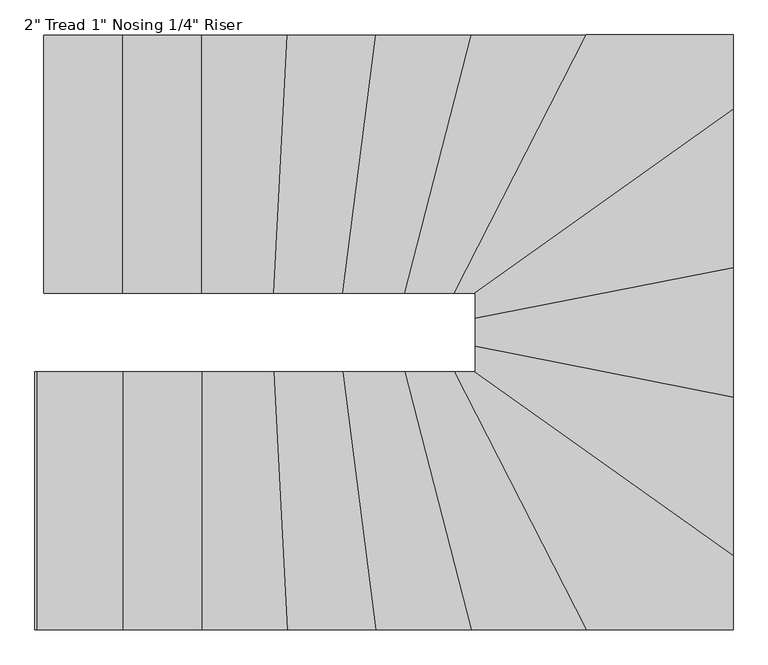
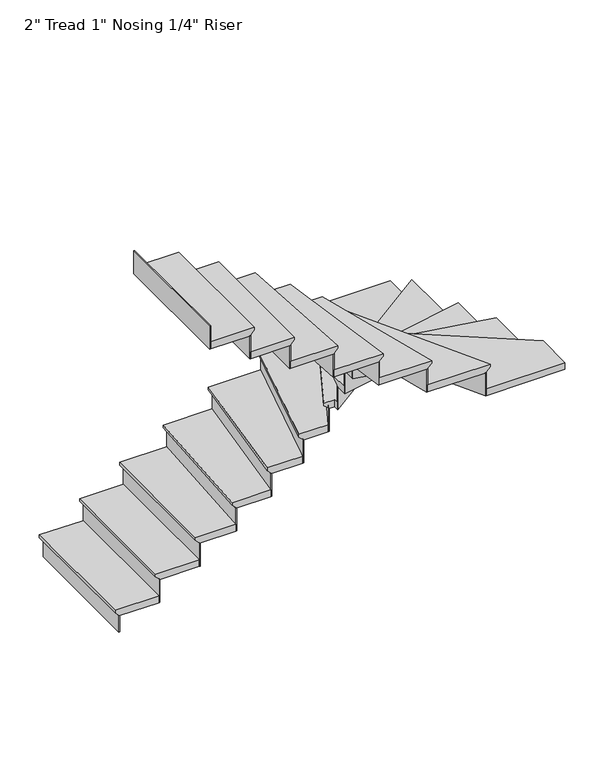
"""IFC4 building model written with IfcOpenShell, lengths in millimetres: stair flight geometry."""

from ifc_helpers import new_model, si_unit, origin, place, context, project, spatial, faceted_brep, source, transform, mapped, element, save


def stair_flight_cbf97d32(model_context):
    return source(origin(), model_context, "Body", "Brep", [
        faceted_brep([(-7803.5154882, 6201.5759458, 150.2833333), (-7803.5154882, 6201.5759458, 169.3333333), (-7803.5154882, 7115.9759458, 169.3333333), (-7803.5154882, 7115.9759458, 150.2833333), (-7778.1154882, 6201.5759458, 124.8833333), (-7778.1154882, 7115.9759458, 124.8833333), (-7498.7154882, 6201.5759458, 169.3333333), (-7498.7154882, 7115.9759458, 169.3333333), (-7778.1154882, 7115.9759458, 118.5333333), (-7498.7154882, 7115.9759458, 118.5333333), (-7498.7154882, 6201.5759458, 118.5333333), (-7778.1154882, 6201.5759458, 118.5333333)], [[[0, 1, 2, 3]], [[4, 0, 3, 5]], [[2, 1, 6, 7]], [[8, 9, 10, 11]], [[2, 7, 9, 8, 5, 3]], [[8, 11, 4, 5]], [[6, 1, 0, 4, 11, 10]], [[7, 6, 10, 9]]]),
        faceted_brep([(-7778.1154882, 6201.5759458, 118.5333333), (-7778.1154882, 6201.5759458, 0.0), (-7771.7654882, 6201.5759458, 0.0), (-7771.7654882, 6201.5759458, 118.5333333), (-7778.1154882, 7115.9759458, 118.5333333), (-7771.7654882, 7115.9759458, 118.5333333), (-7771.7654882, 7115.9759458, 0.0), (-7778.1154882, 7115.9759458, 0.0)], [[[0, 1, 2, 3]], [[4, 5, 6, 7]], [[1, 0, 4, 7]], [[2, 1, 7, 6]], [[3, 2, 6, 5]], [[0, 3, 5, 4]]]),
        faceted_brep([(-7498.7154882, 6201.5759458, 287.8666667), (-7498.7154882, 6201.5759458, 118.5333333), (-7492.3654882, 6201.5759458, 118.5333333), (-7492.3654882, 6201.5759458, 287.8666667), (-7498.7154882, 7115.9759458, 287.8666667), (-7492.3654882, 7115.9759458, 287.8666667), (-7492.3654882, 7115.9759458, 118.5333333), (-7498.7154882, 7115.9759458, 118.5333333)], [[[0, 1, 2, 3]], [[4, 5, 6, 7]], [[1, 0, 4, 7]], [[2, 1, 7, 6]], [[3, 2, 6, 5]], [[0, 3, 5, 4]]]),
        faceted_brep([(-7524.1154882, 7115.9759458, 338.6666667), (-7524.1154882, 6201.5759458, 338.6666667), (-7219.3154882, 6201.5759458, 338.6666667), (-7219.3154882, 7115.9759458, 338.6666667), (-7498.7154882, 7115.9759458, 287.8666667), (-7219.3154882, 7115.9759458, 287.8666667), (-7219.3154882, 6201.5759458, 287.8666667), (-7498.7154882, 6201.5759458, 287.8666667), (-7498.7154882, 7115.9759458, 294.2166667), (-7524.1154882, 7115.9759458, 319.6166667), (-7498.7154882, 6201.5759458, 294.2166667), (-7524.1154882, 6201.5759458, 319.6166667)], [[[0, 1, 2, 3]], [[4, 5, 6, 7]], [[0, 3, 5, 4, 8, 9]], [[4, 7, 10, 8]], [[2, 1, 11, 10, 7, 6]], [[3, 2, 6, 5]], [[11, 1, 0, 9]], [[10, 11, 9, 8]]]),
        faceted_brep([(-7219.3154882, 6201.5759458, 457.2), (-7219.3154882, 6201.5759458, 287.8666667), (-7212.9654882, 6201.5759458, 287.8666667), (-7212.9654882, 6201.5759458, 457.2), (-7219.3154882, 7115.9759458, 457.2), (-7212.9654882, 7115.9759458, 457.2), (-7212.9654882, 7115.9759458, 287.8666667), (-7219.3154882, 7115.9759458, 287.8666667)], [[[0, 1, 2, 3]], [[4, 5, 6, 7]], [[1, 0, 4, 7]], [[2, 1, 7, 6]], [[3, 2, 6, 5]], [[0, 3, 5, 4]]]),
        faceted_brep([(-7244.7154882, 7115.9759458, 508.0), (-7244.7154882, 6201.5759458, 508.0), (-6963.6483268, 6201.5759458, 508.0), (-6916.1140564, 7115.9759458, 508.0), (-7219.3154882, 7115.9759458, 457.2), (-6916.1140564, 7115.9759458, 457.2), (-6963.6483268, 6201.5759458, 457.2), (-7219.3154882, 6201.5759458, 457.2), (-7219.3154882, 7115.9759458, 463.55), (-7244.7154882, 7115.9759458, 488.95), (-7219.3154882, 6201.5759458, 463.55), (-7244.7154882, 6201.5759458, 488.95)], [[[0, 1, 2, 3]], [[4, 5, 6, 7]], [[0, 3, 5, 4, 8, 9]], [[4, 7, 10, 8]], [[2, 1, 11, 10, 7, 6]], [[3, 2, 6, 5]], [[11, 1, 0, 9]], [[10, 11, 9, 8]]]),
        faceted_brep([(-6963.6483268, 6201.5759458, 626.5333333), (-6963.6483268, 6201.5759458, 457.2), (-6957.2897526, 6201.5759458, 457.2), (-6957.2897526, 6201.5759458, 626.5333333), (-6916.1140564, 7115.9759458, 626.5333333), (-6909.7554822, 7115.9759458, 626.5333333), (-6909.7554822, 7115.9759458, 457.2), (-6916.1140564, 7115.9759458, 457.2)], [[[0, 1, 2, 3]], [[4, 5, 6, 7]], [[1, 0, 4, 7]], [[2, 1, 7, 6]], [[3, 2, 6, 5]], [[0, 3, 5, 4]]]),
        faceted_brep([(-6941.548353, 7115.9759458, 677.3333333), (-6989.0826234, 6201.5759458, 677.3333333), (-6719.4816269, 6201.5759458, 677.3333333), (-6601.1255753, 7115.9759458, 677.3333333), (-6916.1140564, 7115.9759458, 626.5333333), (-6601.1255753, 7115.9759458, 626.5333333), (-6719.4816269, 6201.5759458, 626.5333333), (-6963.6483268, 6201.5759458, 626.5333333), (-6916.1140564, 7115.9759458, 632.8833333), (-6941.548353, 7115.9759458, 658.2833333), (-6963.6483268, 6201.5759458, 632.8833333), (-6989.0826234, 6201.5759458, 658.2833333)], [[[0, 1, 2, 3]], [[4, 5, 6, 7]], [[0, 3, 5, 4, 8, 9]], [[4, 7, 10, 8]], [[2, 1, 11, 10, 7, 6]], [[3, 2, 6, 5]], [[11, 1, 0, 9]], [[10, 11, 9, 8]]]),
        faceted_brep([(-6719.4816269, 6201.5759458, 795.8666667), (-6719.4816269, 6201.5759458, 626.5333333), (-6713.0786552, 6201.5759458, 626.5333333), (-6713.0786552, 6201.5759458, 795.8666667), (-6601.1255753, 7115.9759458, 795.8666667), (-6594.7226035, 7115.9759458, 795.8666667), (-6594.7226035, 7115.9759458, 626.5333333), (-6601.1255753, 7115.9759458, 626.5333333)], [[[0, 1, 2, 3]], [[4, 5, 6, 7]], [[1, 0, 4, 7]], [[2, 1, 7, 6]], [[3, 2, 6, 5]], [[0, 3, 5, 4]]]),
        faceted_brep([(-6626.7374624, 7115.9759458, 846.6666667), (-6745.0935141, 6201.5759458, 846.6666667), (-6497.8544045, 6201.5759458, 846.6666667), (-6262.7239571, 7115.9759458, 846.6666667), (-6601.1255753, 7115.9759458, 795.8666667), (-6262.7239571, 7115.9759458, 795.8666667), (-6497.8544045, 6201.5759458, 795.8666667), (-6719.4816269, 6201.5759458, 795.8666667), (-6601.1255753, 7115.9759458, 802.2166667), (-6626.7374624, 7115.9759458, 827.6166667), (-6719.4816269, 6201.5759458, 802.2166667), (-6745.0935141, 6201.5759458, 827.6166667)], [[[0, 1, 2, 3]], [[4, 5, 6, 7]], [[0, 3, 5, 4, 8, 9]], [[4, 7, 10, 8]], [[2, 1, 11, 10, 7, 6]], [[3, 2, 6, 5]], [[11, 1, 0, 9]], [[10, 11, 9, 8]]]),
        faceted_brep([(-6497.8544045, 6201.5759458, 965.2), (-6497.8544045, 6201.5759458, 795.8666667), (-6491.2978276, 6201.5759458, 795.8666667), (-6491.2978276, 6201.5759458, 965.2), (-6262.7239571, 7115.9759458, 965.2), (-6256.1673802, 7115.9759458, 965.2), (-6256.1673802, 7115.9759458, 795.8666667), (-6262.7239571, 7115.9759458, 795.8666667)], [[[0, 1, 2, 3]], [[4, 5, 6, 7]], [[1, 0, 4, 7]], [[2, 1, 7, 6]], [[3, 2, 6, 5]], [[0, 3, 5, 4]]]),
        faceted_brep([(-6288.9502645, 7115.9759458, 1016.0), (-6524.0807119, 6201.5759458, 1016.0), (-6321.5077684, 6201.5759458, 1016.0), (-5852.6831471, 7115.9759458, 1016.0), (-6262.7239571, 7115.9759458, 965.2), (-5852.6831471, 7115.9759458, 965.2), (-6321.5077684, 6201.5759458, 965.2), (-6497.8544045, 6201.5759458, 965.2), (-6262.7239571, 7115.9759458, 971.55), (-6288.9502645, 7115.9759458, 996.95), (-6497.8544045, 6201.5759458, 971.55), (-6524.0807119, 6201.5759458, 996.95)], [[[0, 1, 2, 3]], [[4, 5, 6, 7]], [[0, 3, 5, 4, 8, 9]], [[4, 7, 10, 8]], [[2, 1, 11, 10, 7, 6]], [[3, 2, 6, 5]], [[11, 1, 0, 9]], [[10, 11, 9, 8]]]),
        faceted_brep([(-6321.5077684, 6201.5759458, 1134.5333333), (-6321.5077684, 6201.5759458, 965.2), (-6314.3717853, 6201.5759458, 965.2), (-6314.3717853, 6201.5759458, 1134.5333333), (-5852.6831471, 7115.9759458, 1134.5333333), (-5845.5471639, 7115.9759458, 1134.5333333), (-5845.5471639, 7115.9759458, 965.2), (-5852.6831471, 7115.9759458, 965.2)], [[[0, 1, 2, 3]], [[4, 5, 6, 7]], [[1, 0, 4, 7]], [[2, 1, 7, 6]], [[3, 2, 6, 5]], [[0, 3, 5, 4]]]),
        faceted_brep([(-5361.3837964, 6822.2948121, 1185.3333333), (-5361.3837964, 7115.9759458, 1185.3333333), (-5881.2270796, 7115.9759458, 1185.3333333), (-6350.0517009, 6201.5759458, 1185.3333333), (-6275.7837964, 6201.5759458, 1185.3333333), (-6275.7837964, 6172.020863, 1185.3333333), (-5361.3837964, 7115.9759458, 1134.5333333), (-5361.3837964, 6822.2948121, 1134.5333333), (-6275.7837964, 6172.020863, 1134.5333333), (-6275.7837964, 6201.5759458, 1134.5333333), (-6321.5077684, 6201.5759458, 1134.5333333), (-5852.6831471, 7115.9759458, 1134.5333333), (-5852.6831471, 7115.9759458, 1140.8833333), (-5881.2270796, 7115.9759458, 1166.2833333), (-6321.5077684, 6201.5759458, 1140.8833333), (-6350.0517009, 6201.5759458, 1166.2833333)], [[[0, 1, 2, 3, 4, 5]], [[6, 7, 8, 9, 10, 11]], [[1, 0, 7, 6]], [[2, 1, 6, 11, 12, 13]], [[11, 10, 14, 12]], [[4, 3, 15, 14, 10, 9]], [[5, 4, 9, 8]], [[0, 5, 8, 7]], [[15, 3, 2, 13]], [[14, 15, 13, 12]]]),
        faceted_brep([(-6275.7837964, 6172.020863, 1303.8666667), (-6275.7837964, 6172.020863, 1134.5333333), (-6275.7837964, 6164.2288882, 1134.5333333), (-6275.7837964, 6164.2288882, 1303.8666667), (-5361.3837964, 6822.2948121, 1303.8666667), (-5361.3837964, 6814.5028373, 1303.8666667), (-5361.3837964, 6814.5028373, 1134.5333333), (-5361.3837964, 6822.2948121, 1134.5333333)], [[[0, 1, 2, 3]], [[4, 5, 6, 7]], [[1, 0, 4, 7]], [[2, 1, 7, 6]], [[3, 2, 6, 5]], [[0, 3, 5, 4]]]),
        faceted_brep([(-5361.3837964, 6853.4627113, 1354.6666667), (-6275.7837964, 6203.1887621, 1354.6666667), (-6275.7837964, 6085.5667759, 1354.6666667), (-5361.3837964, 6265.8076322, 1354.6666667), (-5361.3837964, 6822.2948121, 1303.8666667), (-5361.3837964, 6265.8076322, 1303.8666667), (-6275.7837964, 6085.5667759, 1303.8666667), (-6275.7837964, 6172.020863, 1303.8666667), (-5361.3837964, 6822.2948121, 1310.2166667), (-5361.3837964, 6853.4627113, 1335.6166667), (-6275.7837964, 6172.020863, 1310.2166667), (-6275.7837964, 6203.1887621, 1335.6166667)], [[[0, 1, 2, 3]], [[4, 5, 6, 7]], [[0, 3, 5, 4, 8, 9]], [[4, 7, 10, 8]], [[2, 1, 11, 10, 7, 6]], [[3, 2, 6, 5]], [[11, 1, 0, 9]], [[10, 11, 9, 8]]]),
        faceted_brep([(-6275.7837964, 6085.5667759, 1473.2), (-6275.7837964, 6085.5667759, 1303.8666667), (-6275.7837964, 6079.0945905, 1303.8666667), (-6275.7837964, 6079.0945905, 1473.2), (-5361.3837964, 6265.8076322, 1473.2), (-5361.3837964, 6259.3354468, 1473.2), (-5361.3837964, 6259.3354468, 1303.8666667), (-5361.3837964, 6265.8076322, 1303.8666667)], [[[0, 1, 2, 3]], [[4, 5, 6, 7]], [[1, 0, 4, 7]], [[2, 1, 7, 6]], [[3, 2, 6, 5]], [[0, 3, 5, 4]]]),
        faceted_brep([(-5361.3837964, 6291.696374, 1524.0), (-6275.7837964, 6111.4555176, 1524.0), (-6275.7837964, 5986.4076322, 1524.0), (-5361.3837964, 5806.1667759, 1524.0), (-5361.3837964, 6265.8076322, 1473.2), (-5361.3837964, 5806.1667759, 1473.2), (-6275.7837964, 5986.4076322, 1473.2), (-6275.7837964, 6085.5667759, 1473.2), (-5361.3837964, 6265.8076322, 1479.55), (-5361.3837964, 6291.696374, 1504.95), (-6275.7837964, 6085.5667759, 1479.55), (-6275.7837964, 6111.4555176, 1504.95)], [[[0, 1, 2, 3]], [[4, 5, 6, 7]], [[0, 3, 5, 4, 8, 9]], [[4, 7, 10, 8]], [[2, 1, 11, 10, 7, 6]], [[3, 2, 6, 5]], [[11, 1, 0, 9]], [[10, 11, 9, 8]]]),
        faceted_brep([(-6275.7837964, 5986.4076322, 1642.5333333), (-6275.7837964, 5986.4076322, 1473.2), (-6275.7837964, 5979.9354468, 1473.2), (-6275.7837964, 5979.9354468, 1642.5333333), (-5361.3837964, 5806.1667759, 1642.5333333), (-5361.3837964, 5799.6945905, 1642.5333333), (-5361.3837964, 5799.6945905, 1473.2), (-5361.3837964, 5806.1667759, 1473.2)], [[[0, 1, 2, 3]], [[4, 5, 6, 7]], [[1, 0, 4, 7]], [[2, 1, 7, 6]], [[3, 2, 6, 5]], [[0, 3, 5, 4]]]),
        faceted_brep([(-5361.3837964, 5832.0555176, 1693.3333333), (-6275.7837964, 6012.296374, 1693.3333333), (-6275.7837964, 5922.1759458, 1693.3333333), (-6321.8792709, 5922.1759458, 1693.3333333), (-5361.3837964, 5239.1212812, 1693.3333333), (-5361.3837964, 5806.1667759, 1642.5333333), (-5361.3837964, 5239.1212812, 1642.5333333), (-6321.8792709, 5922.1759458, 1642.5333333), (-6275.7837964, 5922.1759458, 1642.5333333), (-6275.7837964, 5986.4076322, 1642.5333333), (-5361.3837964, 5806.1667759, 1648.8833333), (-5361.3837964, 5832.0555176, 1674.2833333), (-6275.7837964, 5986.4076322, 1648.8833333), (-6275.7837964, 6012.296374, 1674.2833333)], [[[0, 1, 2, 3, 4]], [[5, 6, 7, 8, 9]], [[0, 4, 6, 5, 10, 11]], [[5, 9, 12, 10]], [[2, 1, 13, 12, 9, 8]], [[3, 2, 8, 7]], [[4, 3, 7, 6]], [[13, 1, 0, 11]], [[12, 13, 11, 10]]]),
        faceted_brep([(-6321.8792709, 5922.1759458, 1811.8666667), (-6321.8792709, 5922.1759458, 1642.5333333), (-6332.8361634, 5922.1759458, 1642.5333333), (-6332.8361634, 5922.1759458, 1811.8666667), (-5361.3837964, 5239.1212812, 1811.8666667), (-5361.3837964, 5231.3293064, 1811.8666667), (-5361.3837964, 5231.3293064, 1642.5333333), (-5361.3837964, 5239.1212812, 1642.5333333)], [[[0, 1, 2, 3]], [[4, 5, 6, 7]], [[1, 0, 4, 7]], [[2, 1, 7, 6]], [[3, 2, 6, 5]], [[0, 3, 5, 4]]]),
        faceted_brep([(-5909.7710121, 5007.7759458, 1862.6666667), (-5361.3837964, 5007.7759458, 1862.6666667), (-5361.3837964, 5270.2891803, 1862.6666667), (-6278.0517009, 5922.1759458, 1862.6666667), (-6378.5956335, 5922.1759458, 1862.6666667), (-5361.3837964, 5007.7759458, 1811.8666667), (-5909.7710121, 5007.7759458, 1811.8666667), (-6378.5956335, 5922.1759458, 1811.8666667), (-6321.8792709, 5922.1759458, 1811.8666667), (-5361.3837964, 5239.1212812, 1811.8666667), (-5361.3837964, 5239.1212812, 1818.2166667), (-5361.3837964, 5270.2891803, 1843.6166667), (-6321.8792709, 5922.1759458, 1818.2166667), (-6278.0517009, 5922.1759458, 1843.6166667)], [[[0, 1, 2, 3, 4]], [[5, 6, 7, 8, 9]], [[1, 0, 6, 5]], [[2, 1, 5, 9, 10, 11]], [[9, 8, 12, 10]], [[4, 3, 13, 12, 8, 7]], [[0, 4, 7, 6]], [[13, 3, 2, 11]], [[12, 13, 11, 10]]]),
        faceted_brep([(-6378.5956335, 5922.1759458, 1981.2), (-6378.5956335, 5922.1759458, 1811.8666667), (-6385.7316166, 5922.1759458, 1811.8666667), (-6385.7316166, 5922.1759458, 1981.2), (-5909.7710121, 5007.7759458, 1981.2), (-5916.9069953, 5007.7759458, 1981.2), (-5916.9069953, 5007.7759458, 1811.8666667), (-5909.7710121, 5007.7759458, 1811.8666667)], [[[0, 1, 2, 3]], [[4, 5, 6, 7]], [[1, 0, 4, 7]], [[2, 1, 7, 6]], [[3, 2, 6, 5]], [[0, 3, 5, 4]]]),
        faceted_brep([(-5881.2270796, 5007.7759458, 2032.0), (-6350.0517009, 5922.1759458, 2032.0), (-6550.3070194, 5922.1759458, 2032.0), (-6315.176572, 5007.7759458, 2032.0), (-5909.7710121, 5007.7759458, 1981.2), (-6315.176572, 5007.7759458, 1981.2), (-6550.3070194, 5922.1759458, 1981.2), (-6378.5956335, 5922.1759458, 1981.2), (-5909.7710121, 5007.7759458, 1987.55), (-5881.2270796, 5007.7759458, 2012.95), (-6378.5956335, 5922.1759458, 1987.55), (-6350.0517009, 5922.1759458, 2012.95)], [[[0, 1, 2, 3]], [[4, 5, 6, 7]], [[0, 3, 5, 4, 8, 9]], [[4, 7, 10, 8]], [[2, 1, 11, 10, 7, 6]], [[3, 2, 6, 5]], [[11, 1, 0, 9]], [[10, 11, 9, 8]]]),
        faceted_brep([(-6550.3070194, 5922.1759458, 2150.5333333), (-6550.3070194, 5922.1759458, 1981.2), (-6556.8635963, 5922.1759458, 1981.2), (-6556.8635963, 5922.1759458, 2150.5333333), (-6315.176572, 5007.7759458, 2150.5333333), (-6321.7331489, 5007.7759458, 2150.5333333), (-6321.7331489, 5007.7759458, 1981.2), (-6315.176572, 5007.7759458, 1981.2)], [[[0, 1, 2, 3]], [[4, 5, 6, 7]], [[1, 0, 4, 7]], [[2, 1, 7, 6]], [[3, 2, 6, 5]], [[0, 3, 5, 4]]]),
        faceted_brep([(-6288.9502645, 5007.7759458, 2201.3333333), (-6524.0807119, 5922.1759458, 2201.3333333), (-6770.7054012, 5922.1759458, 2201.3333333), (-6652.3493495, 5007.7759458, 2201.3333333), (-6315.176572, 5007.7759458, 2150.5333333), (-6652.3493495, 5007.7759458, 2150.5333333), (-6770.7054012, 5922.1759458, 2150.5333333), (-6550.3070194, 5922.1759458, 2150.5333333), (-6315.176572, 5007.7759458, 2156.8833333), (-6288.9502645, 5007.7759458, 2182.2833333), (-6550.3070194, 5922.1759458, 2156.8833333), (-6524.0807119, 5922.1759458, 2182.2833333)], [[[0, 1, 2, 3]], [[4, 5, 6, 7]], [[0, 3, 5, 4, 8, 9]], [[4, 7, 10, 8]], [[2, 1, 11, 10, 7, 6]], [[3, 2, 6, 5]], [[11, 1, 0, 9]], [[10, 11, 9, 8]]]),
        faceted_brep([(-6770.7054012, 5922.1759458, 2319.8666667), (-6770.7054012, 5922.1759458, 2150.5333333), (-6777.108373, 5922.1759458, 2150.5333333), (-6777.108373, 5922.1759458, 2319.8666667), (-6652.3493495, 5007.7759458, 2319.8666667), (-6658.7523213, 5007.7759458, 2319.8666667), (-6658.7523213, 5007.7759458, 2150.5333333), (-6652.3493495, 5007.7759458, 2150.5333333)], [[[0, 1, 2, 3]], [[4, 5, 6, 7]], [[1, 0, 4, 7]], [[2, 1, 7, 6]], [[3, 2, 6, 5]], [[0, 3, 5, 4]]]),
        faceted_brep([(-6626.7374624, 5007.7759458, 2370.6666667), (-6745.0935141, 5922.1759458, 2370.6666667), (-7014.5169201, 5922.1759458, 2370.6666667), (-6966.9826497, 5007.7759458, 2370.6666667), (-6652.3493495, 5007.7759458, 2319.8666667), (-6966.9826497, 5007.7759458, 2319.8666667), (-7014.5169201, 5922.1759458, 2319.8666667), (-6770.7054012, 5922.1759458, 2319.8666667), (-6652.3493495, 5007.7759458, 2326.2166667), (-6626.7374624, 5007.7759458, 2351.6166667), (-6770.7054012, 5922.1759458, 2326.2166667), (-6745.0935141, 5922.1759458, 2351.6166667)], [[[0, 1, 2, 3]], [[4, 5, 6, 7]], [[0, 3, 5, 4, 8, 9]], [[4, 7, 10, 8]], [[2, 1, 11, 10, 7, 6]], [[3, 2, 6, 5]], [[11, 1, 0, 9]], [[10, 11, 9, 8]]]),
        faceted_brep([(-7014.5169201, 5922.1759458, 2489.2), (-7014.5169201, 5922.1759458, 2319.8666667), (-7020.8754943, 5922.1759458, 2319.8666667), (-7020.8754943, 5922.1759458, 2489.2), (-6966.9826497, 5007.7759458, 2489.2), (-6973.3412239, 5007.7759458, 2489.2), (-6973.3412239, 5007.7759458, 2319.8666667), (-6966.9826497, 5007.7759458, 2319.8666667)], [[[0, 1, 2, 3]], [[4, 5, 6, 7]], [[1, 0, 4, 7]], [[2, 1, 7, 6]], [[3, 2, 6, 5]], [[0, 3, 5, 4]]]),
        faceted_brep([(-6941.548353, 5007.7759458, 2540.0), (-6989.0826234, 5922.1759458, 2540.0), (-7270.1154882, 5922.1759458, 2540.0), (-7270.1154882, 5007.7759458, 2540.0), (-6966.9826497, 5007.7759458, 2489.2), (-7270.1154882, 5007.7759458, 2489.2), (-7270.1154882, 5922.1759458, 2489.2), (-7014.5169201, 5922.1759458, 2489.2), (-6966.9826497, 5007.7759458, 2495.55), (-6941.548353, 5007.7759458, 2520.95), (-7014.5169201, 5922.1759458, 2495.55), (-6989.0826234, 5922.1759458, 2520.95)], [[[0, 1, 2, 3]], [[4, 5, 6, 7]], [[0, 3, 5, 4, 8, 9]], [[4, 7, 10, 8]], [[2, 1, 11, 10, 7, 6]], [[3, 2, 6, 5]], [[11, 1, 0, 9]], [[10, 11, 9, 8]]]),
        faceted_brep([(-7270.1154882, 5922.1759458, 2658.5333333), (-7270.1154882, 5922.1759458, 2489.2), (-7276.4654882, 5922.1759458, 2489.2), (-7276.4654882, 5922.1759458, 2658.5333333), (-7270.1154882, 5007.7759458, 2658.5333333), (-7276.4654882, 5007.7759458, 2658.5333333), (-7276.4654882, 5007.7759458, 2489.2), (-7270.1154882, 5007.7759458, 2489.2)], [[[0, 1, 2, 3]], [[4, 5, 6, 7]], [[1, 0, 4, 7]], [[2, 1, 7, 6]], [[3, 2, 6, 5]], [[0, 3, 5, 4]]]),
        faceted_brep([(-7244.7154882, 5007.7759458, 2709.3333333), (-7244.7154882, 5922.1759458, 2709.3333333), (-7549.5154882, 5922.1759458, 2709.3333333), (-7549.5154882, 5007.7759458, 2709.3333333), (-7270.1154882, 5007.7759458, 2658.5333333), (-7549.5154882, 5007.7759458, 2658.5333333), (-7549.5154882, 5922.1759458, 2658.5333333), (-7270.1154882, 5922.1759458, 2658.5333333), (-7270.1154882, 5007.7759458, 2664.8833333), (-7244.7154882, 5007.7759458, 2690.2833333), (-7270.1154882, 5922.1759458, 2664.8833333), (-7244.7154882, 5922.1759458, 2690.2833333)], [[[0, 1, 2, 3]], [[4, 5, 6, 7]], [[0, 3, 5, 4, 8, 9]], [[4, 7, 10, 8]], [[2, 1, 11, 10, 7, 6]], [[3, 2, 6, 5]], [[11, 1, 0, 9]], [[10, 11, 9, 8]]]),
        faceted_brep([(-7549.5154882, 5922.1759458, 2827.8666667), (-7549.5154882, 5922.1759458, 2658.5333333), (-7555.8654882, 5922.1759458, 2658.5333333), (-7555.8654882, 5922.1759458, 2827.8666667), (-7549.5154882, 5007.7759458, 2827.8666667), (-7555.8654882, 5007.7759458, 2827.8666667), (-7555.8654882, 5007.7759458, 2658.5333333), (-7549.5154882, 5007.7759458, 2658.5333333)], [[[0, 1, 2, 3]], [[4, 5, 6, 7]], [[1, 0, 4, 7]], [[2, 1, 7, 6]], [[3, 2, 6, 5]], [[0, 3, 5, 4]]]),
        faceted_brep([(-7828.9154882, 5922.1759458, 2997.2), (-7828.9154882, 5922.1759458, 2827.8666667), (-7835.2654882, 5922.1759458, 2827.8666667), (-7835.2654882, 5922.1759458, 2997.2), (-7828.9154882, 5007.7759458, 2997.2), (-7835.2654882, 5007.7759458, 2997.2), (-7835.2654882, 5007.7759458, 2827.8666667), (-7828.9154882, 5007.7759458, 2827.8666667)], [[[0, 1, 2, 3]], [[4, 5, 6, 7]], [[1, 0, 4, 7]], [[2, 1, 7, 6]], [[3, 2, 6, 5]], [[0, 3, 5, 4]]]),
        faceted_brep([(-7524.1154882, 5007.7759458, 2878.6666667), (-7524.1154882, 5922.1759458, 2878.6666667), (-7828.9154882, 5922.1759458, 2878.6666667), (-7828.9154882, 5007.7759458, 2878.6666667), (-7549.5154882, 5007.7759458, 2827.8666667), (-7828.9154882, 5007.7759458, 2827.8666667), (-7828.9154882, 5922.1759458, 2827.8666667), (-7549.5154882, 5922.1759458, 2827.8666667), (-7549.5154882, 5007.7759458, 2834.2166667), (-7524.1154882, 5007.7759458, 2859.6166667), (-7549.5154882, 5922.1759458, 2834.2166667), (-7524.1154882, 5922.1759458, 2859.6166667)], [[[0, 1, 2, 3]], [[4, 5, 6, 7]], [[0, 3, 5, 4, 8, 9]], [[4, 7, 10, 8]], [[2, 1, 11, 10, 7, 6]], [[3, 2, 6, 5]], [[11, 1, 0, 9]], [[10, 11, 9, 8]]]),
    ])


if __name__ == "__main__":
    model = new_model("IFC4")
    model_context = context("Model", 3, world=origin())
    ifc_project = project(units=[si_unit("LENGTHUNIT", "METRE", prefix="MILLI")], contexts=[model_context])
    site = spatial("IfcSite", under=ifc_project)
    building = spatial("IfcBuilding", under=site)
    placement = place(None, origin())
    stair_flight_shape = stair_flight_cbf97d32(model_context)
    element("IfcStairFlight", 1, ObjectType="2\" Tread 1\" Nosing 1/4\" Riser", at=placement, inside=building, context=model_context, shape_type="MappedRepresentation", body=[
        mapped(stair_flight_shape, transform((0.0, 0.0, 0.0), x_axis=(1.0, 0.0, 0.0), y_axis=(0.0, 1.0, 0.0), z_axis=(0.0, 0.0, 1.0))),
    ])
    save(model, "model.ifc")
